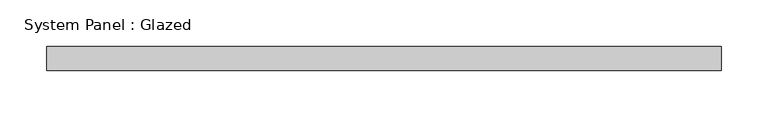
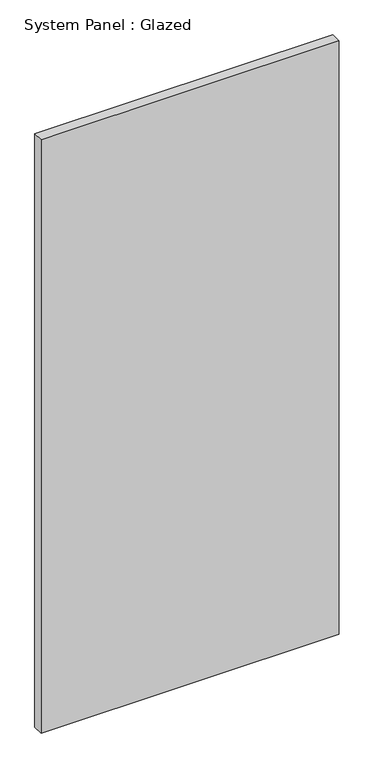
"""IFC4 building model written with IfcOpenShell, lengths in millimetres: plate geometry, System Panel : Glazed."""

from ifc_helpers import new_model, si_unit, origin, origin_with_axes, place, context, project, spatial, polyline, outline, extrude, source, transform, mapped, element, save


def system_panel_glazed_535565c7(model_context):
    return source(origin(), model_context, "Body", "SweptSolid", [
        extrude(outline(polyline([(358.775, 19.05), (-358.775, 19.05), (-358.775, 44.45), (358.775, 44.45), (358.775, 19.05)])), origin_with_axes(), (0.0, 0.0, 1.0), 1509.844519),
    ])


if __name__ == "__main__":
    model = new_model("IFC4")
    model_context = context("Model", 3, world=origin())
    ifc_project = project(units=[si_unit("LENGTHUNIT", "METRE", prefix="MILLI")], contexts=[model_context])
    site = spatial("IfcSite", under=ifc_project)
    building = spatial("IfcBuilding", under=site)
    placement = place(None, origin())
    system_panel_glazed_shape = system_panel_glazed_535565c7(model_context)
    element("IfcPlate", 1, ObjectType="System Panel : Glazed", at=placement, inside=building, context=model_context, shape_type="MappedRepresentation", body=[
        mapped(system_panel_glazed_shape, transform((0.0, 0.0, 0.0), x_axis=(1.0, 0.0, 0.0), y_axis=(0.0, 1.0, 0.0), z_axis=(0.0, 0.0, 1.0))),
    ])
    save(model, "model.ifc")

# Revit data of these elements
# Type "System Panel : Glazed"
#   Construction Type Id = "GSP4R"
#   Analytic Construction = "1/8 in Pilkington single glazing"
#   Visual Light Transmittance = 0.9
#   Solar Heat Gain Coefficient = 0.86
#   Heat Transfer Coefficient (U) = 1.18115 BTU/(h·ft²·°F)
#   Define Thermal Properties by = 1
# Element 1 (IfcPlate, "System Panel : Glazed")
#   Materials on its faces: "Glass"
# Materials
#   "Glass": class "Glass", colour RGB 0 128 192, transparency 0.75, Description = "Soda Lime Glass", Cost = 0
